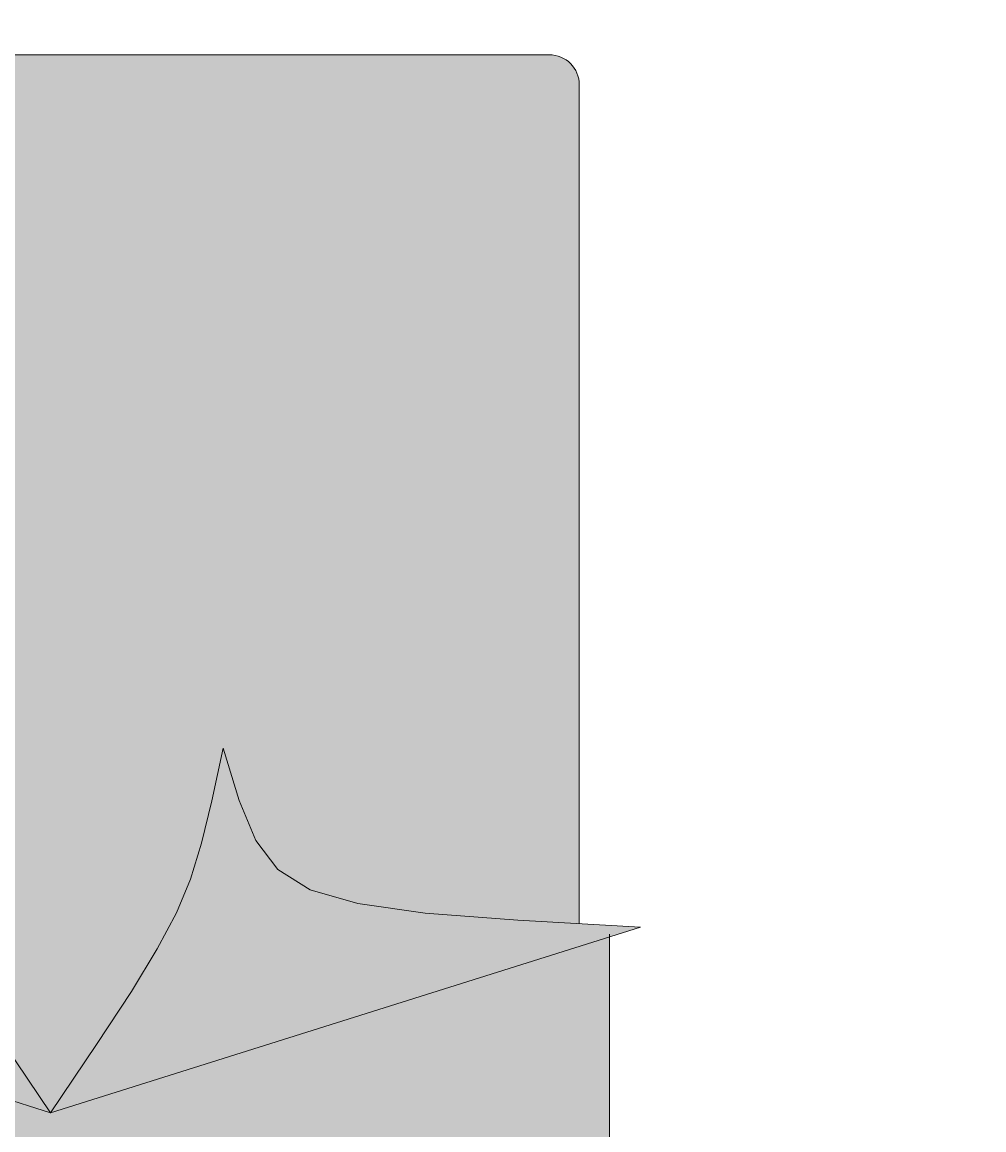
# Model space of a CAD drawing. Units: millimetres. Extents: x 27017497 to 27018854, y 7058029 to 7059154.
# Tile 26 of 91: x 27017702 to 27017753, y 7058163 to 7058222. Entities that reach past the tile are written whole.
import ezdxf

# ---------------------------------------------------------------- set-up
doc = ezdxf.new("R2010")
doc.units = ezdxf.units.MM
doc.layers.add('A-ANNO-DIMS', color=2, linetype='Continuous', lineweight=18)
doc.layers.add('A-FURN', color=8, linetype='Continuous', lineweight=18)
doc.layers.add('A-FURN-PATT', color=177, linetype='Continuous', lineweight=13, true_color=0x293189)
doc.styles.get("Standard").update_dxf_attribs({"font": 'arial.ttf'})
doc.dimstyles.get("Standard").update_dxf_attribs({"dimtxt": 0.18, "dimasz": 0.18, "dimexe": 0.18, "dimexo": 0.0625, "dimgap": 0.09, "dimtad": 0, "dimtih": 1, "dimtoh": 1, "dimdec": 4, "dimzin": 0, "dimdsep": 46, "dimtxsty": 'Standard', "dimcen": 0.09, "dimadec": 0, "dimazin": 0, "dimtfac": 1, "dimtdec": 4, "dimtofl": 0, "dimtmove": 0, "dimatfit": 3, "dimfxl": 1, "dimtolj": 1, "dimtzin": 0, "dimarcsym": 0})

# ---------------------------------------------------------------- blocks, each defined once
blk = doc.blocks.new('CAMMAT')
for p, q in [((-0.6904, -0.5169), (-0.6904, -0.8)), ((0.0535, -0.5623), (-0.7312, -0.8093)), ((0.0535, -0.5623), (0.8382, -0.8093)), ((-0.65, -0.8139), (-0.65, -1.93)), ((0.61, -1.97), (-0.61, -1.97))]:
    blk.add_line(p, q)
for points in [[(-0.1761, -1.0476), (-0.161, -0.9772), (-0.1474, -0.921), (-0.1326, -0.8732), (-0.1139, -0.8282), (-0.0886, -0.7803), (-0.0541, -0.7238), (-0.0076, -0.653), (0.0535, -0.5623)], [(0.2832, -1.0476), (0.2681, -0.9772), (0.2545, -0.921), (0.2396, -0.8732), (0.2209, -0.8282), (0.1957, -0.7803), (0.1611, -0.7238), (0.1147, -0.653), (0.0535, -0.5623)], [(-0.7312, -0.8093), (-0.5683, -0.8185), (-0.4451, -0.828), (-0.3552, -0.8406), (-0.2919, -0.8591), (-0.2489, -0.8862), (-0.2196, -0.9248), (-0.1975, -0.9777), (-0.1761, -1.0476)]]:
    blk.add_lwpolyline(points)
blk.add_arc((-0.61, -1.93), 0.04, 180, 270)
blk = doc.blocks.new('*D47')
at = {"layer": 'A-ANNO-DIMS', "color": 0, "lineweight": -2, "transparency": 16777216}
for p, q in [((27017561.166, 7058294.35), (27017561.166, 7058028.6)), ((27018790.606, 7058294.35), (27018790.606, 7058028.6)), ((27017561.346, 7058028.78), (27018175.431, 7058028.78)), ((27018790.426, 7058028.78), (27018176.341, 7058028.78))]:
    blk.add_line(p, q, dxfattribs=at)
at = {"layer": 'A-ANNO-DIMS', "color": 0, "transparency": 16777216}
for points in [[(27017561.346, 7058028.81), (27017561.346, 7058028.75), (27017561.166, 7058028.78)], [(27018790.426, 7058028.81), (27018790.426, 7058028.75), (27018790.606, 7058028.78)]]:
    blk.add_solid(points, dxfattribs=at)
at = {"layer": 'Defpoints', "color": 0, "transparency": 16777216}
for p in [(27017561.166, 7058294.412), (27018790.606, 7058294.412), (27018790.606, 7058028.78)]:
    blk.add_point(p, dxfattribs=at)
at = {"layer": 'A-ANNO-DIMS', "color": 0, "transparency": 16777216, "insert": (27018175.886, 7058028.78), "char_height": 0.18, "attachment_point": 5}
blk.add_mtext('\\A1;1229.4', dxfattribs=at)
blk = doc.blocks.new('*D48')
at = {"layer": 'A-ANNO-DIMS', "color": 0, "lineweight": -2, "transparency": 16777216}
for p, q in [((27018463.498, 7058622.912), (27017497.536, 7058622.912)), ((27017497.716, 7058622.732), (27017497.716, 7058357.753)), ((27017497.716, 7058092.41), (27017497.716, 7058357.389)), ((27018555.129, 7058092.23), (27017497.536, 7058092.23))]:
    blk.add_line(p, q, dxfattribs=at)
at = {"layer": 'A-ANNO-DIMS', "color": 0, "transparency": 16777216}
for points in [[(27017497.686, 7058622.732), (27017497.746, 7058622.732), (27017497.716, 7058622.912)], [(27017497.686, 7058092.41), (27017497.746, 7058092.41), (27017497.716, 7058092.23)]]:
    blk.add_solid(points, dxfattribs=at)
at = {"layer": 'Defpoints', "color": 0, "transparency": 16777216}
for p in [(27018463.561, 7058622.912), (27017497.716, 7058092.23), (27018555.192, 7058092.23)]:
    blk.add_point(p, dxfattribs=at)
at = {"layer": 'A-ANNO-DIMS', "color": 0, "transparency": 16777216, "insert": (27017497.716, 7058357.571), "char_height": 0.18, "attachment_point": 5}
blk.add_mtext('\\A1;530.7', dxfattribs=at)

msp = doc.modelspace()

# ---------------------------------------------------------------- hatches: boundary and pattern name
at = {"layer": 'A-FURN-PATT'}
h = msp.add_hatch(color=256, dxfattribs=at)
h.dxf.hatch_style = 1
h.paths.add_polyline_path([(27017731.53, 7058218.852, 0.414214), (27017729.937, 7058220.445), (27017681.344, 7058220.445, 0.414214), (27017679.751, 7058218.852), (27017679.751, 7058174.658), (27017683.647, 7058174.959), (27017687.23, 7058175.46), (27017689.748, 7058176.196), (27017691.461, 7058177.277), (27017692.628, 7058178.816), (27017693.508, 7058180.922), (27017694.36, 7058183.707), (27017694.963, 7058180.902), (27017695.506, 7058178.662), (27017696.096, 7058176.759), (27017696.84, 7058174.966), (27017697.847, 7058173.059), (27017699.222, 7058170.809), (27017701.073, 7058167.99), (27017703.508, 7058164.376), (27017705.943, 7058167.99), (27017707.794, 7058170.809), (27017709.169, 7058173.059), (27017710.176, 7058174.966), (27017710.92, 7058176.759), (27017711.51, 7058178.662), (27017712.053, 7058180.902), (27017712.656, 7058183.707), (27017713.508, 7058180.922), (27017714.388, 7058178.816), (27017715.555, 7058177.277), (27017717.268, 7058176.196), (27017719.786, 7058175.46), (27017723.369, 7058174.959), (27017728.274, 7058174.58), (27017731.53, 7058174.396)])
h.paths.add_polyline_path([(27017723.369, 7058174.959), (27017719.786, 7058175.46), (27017717.268, 7058176.196), (27017715.555, 7058177.277), (27017714.388, 7058178.816), (27017713.508, 7058180.922), (27017712.656, 7058183.707), (27017712.053, 7058180.902), (27017711.51, 7058178.662), (27017710.92, 7058176.759), (27017710.176, 7058174.966), (27017709.169, 7058173.059), (27017707.794, 7058170.809), (27017705.943, 7058167.99), (27017703.508, 7058164.376), (27017734.763, 7058174.214), (27017728.274, 7058174.58)])
h.paths.add_polyline_path([(27017696.84, 7058174.966), (27017696.096, 7058176.759), (27017695.506, 7058178.662), (27017694.963, 7058180.902), (27017694.36, 7058183.707), (27017693.508, 7058180.922), (27017692.628, 7058178.816), (27017691.461, 7058177.277), (27017689.748, 7058176.196), (27017687.23, 7058175.46), (27017683.647, 7058174.959), (27017679.751, 7058174.658), (27017678.741, 7058174.58), (27017672.253, 7058174.214), (27017703.508, 7058164.376), (27017701.073, 7058167.99), (27017699.222, 7058170.809), (27017697.847, 7058173.059)])
h.paths.add_polyline_path([(27017678.454, 7058172.262), (27017678.454, 7058162.569), (27017733.139, 7058162.569), (27017733.139, 7058173.703), (27017703.508, 7058164.376)])
h.paths.add_polyline_path([(27017730.145, 7058158.291, 0.41419), (27017728.95, 7058159.485), (27017707.491, 7058159.485, 0.414214), (27017706.296, 7058158.29), (27017706.296, 7058148.731, 0.414214), (27017707.491, 7058147.536), (27017728.95, 7058147.536, 0.414237), (27017730.145, 7058148.731)], flags=0)
h.paths.add_polyline_path([(27017731.53, 7058162.569), (27017679.751, 7058162.569), (27017679.751, 7058146.361, 0.414214), (27017681.344, 7058144.768), (27017729.937, 7058144.768, 0.414214), (27017731.53, 7058146.361)])
h.paths.add_polyline_path([(27017703.354, 7058159.485, -0.41419), (27017704.549, 7058158.291), (27017704.549, 7058148.731, -0.414237), (27017703.354, 7058147.536), (27017681.894, 7058147.536, -0.41419), (27017680.699, 7058148.731), (27017680.699, 7058158.29, -0.414237), (27017681.894, 7058159.485)], flags=0)
h.paths.add_polyline_path([(27017707.491, 7058159.485), (27017728.95, 7058159.485, -0.41419), (27017730.145, 7058158.291), (27017730.145, 7058148.731, -0.414237), (27017728.95, 7058147.536), (27017707.491, 7058147.536, -0.414214), (27017706.296, 7058148.731), (27017706.296, 7058158.29, -0.414214)], flags=16)
h.paths.add_polyline_path([(27017704.549, 7058158.291, 0.41419), (27017703.354, 7058159.485), (27017681.894, 7058159.485, 0.414237), (27017680.699, 7058158.29), (27017680.699, 7058148.731, 0.41419), (27017681.894, 7058147.536), (27017703.354, 7058147.536, 0.414237), (27017704.549, 7058148.731)], flags=16)
h.paths.add_polyline_path([(27017752.64, 7058160.7), (27017732.725, 7058160.7), (27017732.725, 7058144.768), (27017752.64, 7058144.768)])
h.paths.add_polyline_path([(27017748.698, 7058152.101, -1), (27017736.749, 7058152.101, -1)], flags=16)
h.paths.add_polyline_path([(27017746.424, 7058152.101, -1), (27017739.024, 7058152.101, -1)], flags=0)
h.paths.add_polyline_path([(27017678.556, 7058160.7), (27017658.641, 7058160.7), (27017658.641, 7058144.768), (27017678.556, 7058144.768)])
h.paths.add_polyline_path([(27017674.806, 7058152.101, -1), (27017662.857, 7058152.101, -1)], flags=16)
h.paths.add_polyline_path([(27017672.531, 7058152.101, -1), (27017665.131, 7058152.101, -1)], flags=0)

# ---------------------------------------------------------------- block references
at = {"layer": 'A-FURN', "xscale": 39.82996475819422, "yscale": 39.82996475819422, "zscale": 39.82996475819422, "rotation": 180}
msp.add_blockref('CAMMAT', (27017705.64, 7058141.98), dxfattribs=at)

# ---------------------------------------------------------------- dimensions: what is measured, and where the dimension line sits
at = {"layer": 'A-ANNO-DIMS'}
dim = msp.add_linear_dim(base=(27017497.716, 7058092.23), p1=(27018463.561, 7058622.912), p2=(27018555.192, 7058092.23), angle=90, dimstyle='Standard', override={"dimdec": 1, "dimlfac": 1, "dimrnd": 0, "dimzin": 0, "dimdsep": 46, "dimlunit": 2}, dxfattribs=at)
dim.commit()
dim.dimension.update_dxf_attribs({"geometry": '*D48', "text_midpoint": (27017497.716, 7058357.571)})
dim = msp.add_linear_dim(base=(27018790.606, 7058028.78), p1=(27017561.166, 7058294.412), p2=(27018790.606, 7058294.412), dimstyle='Standard', override={"dimdec": 1, "dimlfac": 1, "dimrnd": 0, "dimzin": 0, "dimdsep": 46, "dimlunit": 2}, dxfattribs=at)
dim.commit()
dim.dimension.update_dxf_attribs({"geometry": '*D47', "text_midpoint": (27018175.886, 7058028.78)})

doc.saveas('drawing.dxf')
